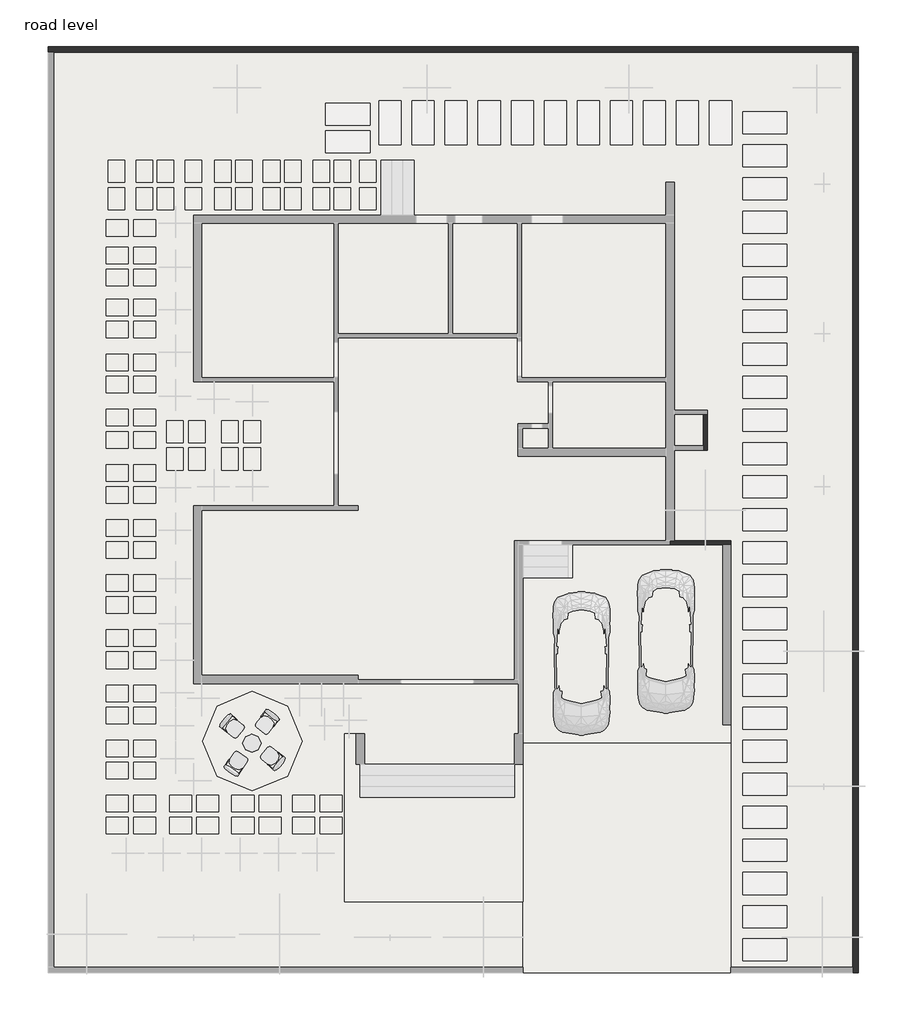
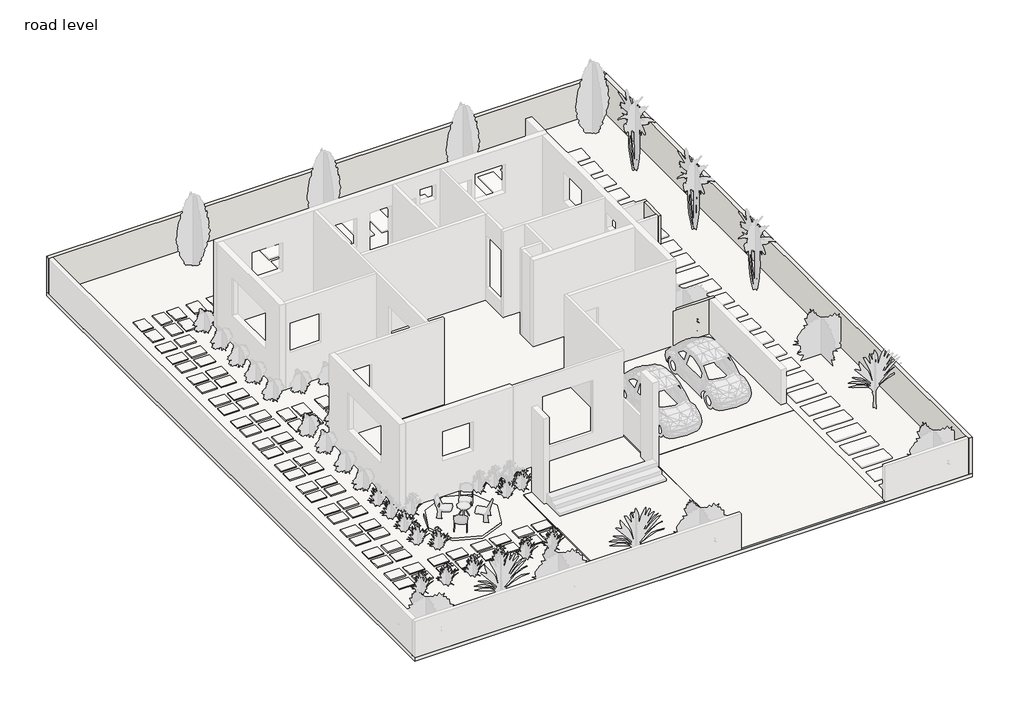
# One storey, part 2 of 3: 6 slabs, 4 walls.
"""IFC4 building model written with IfcOpenShell, lengths in millimetres."""

from ifc_helpers import new_model, si_unit, point, frame, frame_2d, origin, origin_with_axes, place, context, project, spatial, polyline, circle_curve, trimmed, segment, composite_curve, outline, extrude, faceted_brep, element, save

model = new_model("IFC4")

# Units and contexts
model_context = context("Model", 3, world=origin())
ifc_project = project(units=[si_unit("LENGTHUNIT", "METRE", prefix="MILLI")], contexts=[model_context])

# Site, building, storey
site = spatial("IfcSite", under=ifc_project)
building = spatial("IfcBuilding", under=site)
storey = spatial("IfcBuildingStorey", under=building, Name="road level", Elevation=0.0)

# Slabs
placement = place(None, origin())
element("IfcSlab", 1, ObjectType="Generic - 2\"", at=placement, inside=storey, context=model_context, shape_type="SweptSolid", body=[
    extrude(outline(polyline([(-8941.8271365, 12113.4780275), (-8941.8271365, 11503.8780275), (-9399.0271365, 11503.8780275), (-9399.0271365, 12113.4780275), (-8941.8271365, 12113.4780275)])), origin_with_axes(), (0.0, 0.0, 1.0), 50.8),
    extrude(outline(polyline([(-8941.8271365, 11355.5690245), (-8941.8271365, 10745.9690245), (-9399.0271365, 10745.9690245), (-9399.0271365, 11355.5690245), (-8941.8271365, 11355.5690245)])), origin_with_axes(), (0.0, 0.0, 1.0), 50.8),
    extrude(outline(polyline([(-9642.7719122, 12113.4780275), (-9642.7719122, 11503.8780275), (-10099.9719122, 11503.8780275), (-10099.9719122, 12113.4780275), (-9642.7719122, 12113.4780275)])), origin_with_axes(), (0.0, 0.0, 1.0), 50.8),
    extrude(outline(polyline([(-9642.7719122, 11355.5690245), (-9642.7719122, 10745.9690245), (-10099.9719122, 10745.9690245), (-10099.9719122, 11355.5690245), (-9642.7719122, 11355.5690245)])), origin_with_axes(), (0.0, 0.0, 1.0), 50.8),
    extrude(outline(polyline([(-10226.9719122, 12113.4780275), (-10226.9719122, 11503.8780275), (-10684.1719122, 11503.8780275), (-10684.1719122, 12113.4780275), (-10226.9719122, 12113.4780275)])), origin_with_axes(), (0.0, 0.0, 1.0), 50.8),
    extrude(outline(polyline([(-10226.9719122, 11355.5690245), (-10226.9719122, 10745.9690245), (-10684.1719122, 10745.9690245), (-10684.1719122, 11355.5690245), (-10226.9719122, 11355.5690245)])), origin_with_axes(), (0.0, 0.0, 1.0), 50.8),
    extrude(outline(polyline([(-11014.3719122, 12113.4780275), (-11014.3719122, 11503.8780275), (-11471.5719122, 11503.8780275), (-11471.5719122, 12113.4780275), (-11014.3719122, 12113.4780275)])), origin_with_axes(), (0.0, 0.0, 1.0), 50.8),
    extrude(outline(polyline([(-11014.3719122, 11355.5690245), (-11014.3719122, 10745.9690245), (-11471.5719122, 10745.9690245), (-11471.5719122, 11355.5690245), (-11014.3719122, 11355.5690245)])), origin_with_axes(), (0.0, 0.0, 1.0), 50.8),
    extrude(outline(polyline([(-11598.5719122, 12113.4780275), (-11598.5719122, 11503.8780275), (-12055.7719122, 11503.8780275), (-12055.7719122, 12113.4780275), (-11598.5719122, 12113.4780275)])), origin_with_axes(), (0.0, 0.0, 1.0), 50.8),
    extrude(outline(polyline([(-11598.5719122, 11355.5690245), (-11598.5719122, 10745.9690245), (-12055.7719122, 10745.9690245), (-12055.7719122, 11355.5690245), (-11598.5719122, 11355.5690245)])), origin_with_axes(), (0.0, 0.0, 1.0), 50.8),
    extrude(outline(polyline([(-12360.5719122, 12113.4780275), (-12360.5719122, 11503.8780275), (-12817.7719122, 11503.8780275), (-12817.7719122, 12113.4780275), (-12360.5719122, 12113.4780275)])), origin_with_axes(), (0.0, 0.0, 1.0), 50.8),
    extrude(outline(polyline([(-12360.5719122, 11355.5690245), (-12360.5719122, 10745.9690245), (-12817.7719122, 10745.9690245), (-12817.7719122, 11355.5690245), (-12360.5719122, 11355.5690245)])), origin_with_axes(), (0.0, 0.0, 1.0), 50.8),
    extrude(outline(polyline([(-12944.7719122, 12113.4780275), (-12944.7719122, 11503.8780275), (-13401.9719122, 11503.8780275), (-13401.9719122, 12113.4780275), (-12944.7719122, 12113.4780275)])), origin_with_axes(), (0.0, 0.0, 1.0), 50.8),
    extrude(outline(polyline([(-12944.7719122, 11355.5690245), (-12944.7719122, 10745.9690245), (-13401.9719122, 10745.9690245), (-13401.9719122, 11355.5690245), (-12944.7719122, 11355.5690245)])), origin_with_axes(), (0.0, 0.0, 1.0), 50.8),
    extrude(outline(polyline([(-13757.5719122, 12113.4780275), (-13757.5719122, 11503.8780275), (-14214.7719122, 11503.8780275), (-14214.7719122, 12113.4780275), (-13757.5719122, 12113.4780275)])), origin_with_axes(), (0.0, 0.0, 1.0), 50.8),
    extrude(outline(polyline([(-13757.5719122, 11355.5690245), (-13757.5719122, 10745.9690245), (-14214.7719122, 10745.9690245), (-14214.7719122, 11355.5690245), (-13757.5719122, 11355.5690245)])), origin_with_axes(), (0.0, 0.0, 1.0), 50.8),
    extrude(outline(polyline([(-14535.6391446, 12113.4780275), (-14535.6391446, 11503.8780275), (-14992.8391446, 11503.8780275), (-14992.8391446, 12113.4780275), (-14535.6391446, 12113.4780275)])), origin_with_axes(), (0.0, 0.0, 1.0), 50.8),
    extrude(outline(polyline([(-14535.6391446, 11355.5690245), (-14535.6391446, 10745.9690245), (-14992.8391446, 10745.9690245), (-14992.8391446, 11355.5690245), (-14535.6391446, 11355.5690245)])), origin_with_axes(), (0.0, 0.0, 1.0), 50.8),
    extrude(outline(polyline([(-15119.8391446, 12113.4780275), (-15119.8391446, 11503.8780275), (-15577.0391446, 11503.8780275), (-15577.0391446, 12113.4780275), (-15119.8391446, 12113.4780275)])), origin_with_axes(), (0.0, 0.0, 1.0), 50.8),
    extrude(outline(polyline([(-15119.8391446, 11355.5690245), (-15119.8391446, 10745.9690245), (-15577.0391446, 10745.9690245), (-15577.0391446, 11355.5690245), (-15119.8391446, 11355.5690245)])), origin_with_axes(), (0.0, 0.0, 1.0), 50.8),
    extrude(outline(polyline([(-15891.1719122, 12113.4780275), (-15891.1719122, 11503.8780275), (-16348.3719122, 11503.8780275), (-16348.3719122, 12113.4780275), (-15891.1719122, 12113.4780275)])), origin_with_axes(), (0.0, 0.0, 1.0), 50.8),
    extrude(outline(polyline([(-15891.1719122, 11355.5690245), (-15891.1719122, 10745.9690245), (-16348.3719122, 10745.9690245), (-16348.3719122, 11355.5690245), (-15891.1719122, 11355.5690245)])), origin_with_axes(), (0.0, 0.0, 1.0), 50.8),
    extrude(outline(polyline([(-15791.4182051, 10469.9168074), (-15791.4182051, 10012.7168074), (-16401.0182051, 10012.7168074), (-16401.0182051, 10469.9168074), (-15791.4182051, 10469.9168074)])), origin_with_axes(), (0.0, 0.0, 1.0), 50.8),
    extrude(outline(polyline([(-15033.5092021, 10469.9168074), (-15033.5092021, 10012.7168074), (-15643.1092021, 10012.7168074), (-15643.1092021, 10469.9168074), (-15033.5092021, 10469.9168074)])), origin_with_axes(), (0.0, 0.0, 1.0), 50.8),
    extrude(outline(polyline([(-15791.4182051, 9707.9168074), (-15791.4182051, 9250.7168074), (-16401.0182051, 9250.7168074), (-16401.0182051, 9707.9168074), (-15791.4182051, 9707.9168074)])), origin_with_axes(), (0.0, 0.0, 1.0), 50.8),
    extrude(outline(polyline([(-15033.5092021, 9707.9168074), (-15033.5092021, 9250.7168074), (-15643.1092021, 9250.7168074), (-15643.1092021, 9707.9168074), (-15033.5092021, 9707.9168074)])), origin_with_axes(), (0.0, 0.0, 1.0), 50.8),
    extrude(outline(polyline([(-15791.4182051, 9098.3168074), (-15791.4182051, 8641.1168074), (-16401.0182051, 8641.1168074), (-16401.0182051, 9098.3168074), (-15791.4182051, 9098.3168074)])), origin_with_axes(), (0.0, 0.0, 1.0), 50.8),
    extrude(outline(polyline([(-15033.5092021, 9098.3168074), (-15033.5092021, 8641.1168074), (-15643.1092021, 8641.1168074), (-15643.1092021, 9098.3168074), (-15033.5092021, 9098.3168074)])), origin_with_axes(), (0.0, 0.0, 1.0), 50.8),
    extrude(outline(polyline([(-15791.4182051, 8272.8168074), (-15791.4182051, 7815.6168074), (-16401.0182051, 7815.6168074), (-16401.0182051, 8272.8168074), (-15791.4182051, 8272.8168074)])), origin_with_axes(), (0.0, 0.0, 1.0), 50.8),
    extrude(outline(polyline([(-15033.5092021, 8272.8168074), (-15033.5092021, 7815.6168074), (-15643.1092021, 7815.6168074), (-15643.1092021, 8272.8168074), (-15033.5092021, 8272.8168074)])), origin_with_axes(), (0.0, 0.0, 1.0), 50.8),
    extrude(outline(polyline([(-15791.4182051, 7663.2168074), (-15791.4182051, 7206.0168074), (-16401.0182051, 7206.0168074), (-16401.0182051, 7663.2168074), (-15791.4182051, 7663.2168074)])), origin_with_axes(), (0.0, 0.0, 1.0), 50.8),
    extrude(outline(polyline([(-15033.5092021, 7663.2168074), (-15033.5092021, 7206.0168074), (-15643.1092021, 7206.0168074), (-15643.1092021, 7663.2168074), (-15033.5092021, 7663.2168074)])), origin_with_axes(), (0.0, 0.0, 1.0), 50.8),
    extrude(outline(polyline([(-15791.4182051, 6748.8168074), (-15791.4182051, 6291.6168074), (-16401.0182051, 6291.6168074), (-16401.0182051, 6748.8168074), (-15791.4182051, 6748.8168074)])), origin_with_axes(), (0.0, 0.0, 1.0), 50.8),
    extrude(outline(polyline([(-15033.5092021, 6748.8168074), (-15033.5092021, 6291.6168074), (-15643.1092021, 6291.6168074), (-15643.1092021, 6748.8168074), (-15033.5092021, 6748.8168074)])), origin_with_axes(), (0.0, 0.0, 1.0), 50.8),
    extrude(outline(polyline([(-15791.4182051, 6139.2168074), (-15791.4182051, 5682.0168074), (-16401.0182051, 5682.0168074), (-16401.0182051, 6139.2168074), (-15791.4182051, 6139.2168074)])), origin_with_axes(), (0.0, 0.0, 1.0), 50.8),
    extrude(outline(polyline([(-15033.5092021, 6139.2168074), (-15033.5092021, 5682.0168074), (-15643.1092021, 5682.0168074), (-15643.1092021, 6139.2168074), (-15033.5092021, 6139.2168074)])), origin_with_axes(), (0.0, 0.0, 1.0), 50.8),
    extrude(outline(polyline([(-15791.4182051, 5224.8168074), (-15791.4182051, 4767.6168074), (-16401.0182051, 4767.6168074), (-16401.0182051, 5224.8168074), (-15791.4182051, 5224.8168074)])), origin_with_axes(), (0.0, 0.0, 1.0), 50.8),
    extrude(outline(polyline([(-15033.5092021, 5224.8168074), (-15033.5092021, 4767.6168074), (-15643.1092021, 4767.6168074), (-15643.1092021, 5224.8168074), (-15033.5092021, 5224.8168074)])), origin_with_axes(), (0.0, 0.0, 1.0), 50.8),
    extrude(outline(polyline([(-15791.4182051, 4615.2168074), (-15791.4182051, 4158.0168074), (-16401.0182051, 4158.0168074), (-16401.0182051, 4615.2168074), (-15791.4182051, 4615.2168074)])), origin_with_axes(), (0.0, 0.0, 1.0), 50.8),
    extrude(outline(polyline([(-15033.5092021, 4615.2168074), (-15033.5092021, 4158.0168074), (-15643.1092021, 4158.0168074), (-15643.1092021, 4615.2168074), (-15033.5092021, 4615.2168074)])), origin_with_axes(), (0.0, 0.0, 1.0), 50.8),
    extrude(outline(polyline([(-15791.4182051, 3700.8168074), (-15791.4182051, 3243.6168074), (-16401.0182051, 3243.6168074), (-16401.0182051, 3700.8168074), (-15791.4182051, 3700.8168074)])), origin_with_axes(), (0.0, 0.0, 1.0), 50.8),
    extrude(outline(polyline([(-15033.5092021, 3700.8168074), (-15033.5092021, 3243.6168074), (-15643.1092021, 3243.6168074), (-15643.1092021, 3700.8168074), (-15033.5092021, 3700.8168074)])), origin_with_axes(), (0.0, 0.0, 1.0), 50.8),
    extrude(outline(polyline([(-15791.4182051, 3091.2168074), (-15791.4182051, 2634.0168074), (-16401.0182051, 2634.0168074), (-16401.0182051, 3091.2168074), (-15791.4182051, 3091.2168074)])), origin_with_axes(), (0.0, 0.0, 1.0), 50.8),
    extrude(outline(polyline([(-15033.5092021, 3091.2168074), (-15033.5092021, 2634.0168074), (-15643.1092021, 2634.0168074), (-15643.1092021, 3091.2168074), (-15033.5092021, 3091.2168074)])), origin_with_axes(), (0.0, 0.0, 1.0), 50.8),
    extrude(outline(polyline([(-15791.4182051, 2176.8168074), (-15791.4182051, 1719.6168074), (-16401.0182051, 1719.6168074), (-16401.0182051, 2176.8168074), (-15791.4182051, 2176.8168074)])), origin_with_axes(), (0.0, 0.0, 1.0), 50.8),
    extrude(outline(polyline([(-15033.5092021, 2176.8168074), (-15033.5092021, 1719.6168074), (-15643.1092021, 1719.6168074), (-15643.1092021, 2176.8168074), (-15033.5092021, 2176.8168074)])), origin_with_axes(), (0.0, 0.0, 1.0), 50.8),
    extrude(outline(polyline([(-15791.4182051, 1567.2168074), (-15791.4182051, 1110.0168074), (-16401.0182051, 1110.0168074), (-16401.0182051, 1567.2168074), (-15791.4182051, 1567.2168074)])), origin_with_axes(), (0.0, 0.0, 1.0), 50.8),
    extrude(outline(polyline([(-15033.5092021, 1567.2168074), (-15033.5092021, 1110.0168074), (-15643.1092021, 1110.0168074), (-15643.1092021, 1567.2168074), (-15033.5092021, 1567.2168074)])), origin_with_axes(), (0.0, 0.0, 1.0), 50.8),
    extrude(outline(polyline([(-15791.4182051, 652.8168074), (-15791.4182051, 195.6168074), (-16401.0182051, 195.6168074), (-16401.0182051, 652.8168074), (-15791.4182051, 652.8168074)])), origin_with_axes(), (0.0, 0.0, 1.0), 50.8),
    extrude(outline(polyline([(-15033.5092021, 652.8168074), (-15033.5092021, 195.6168074), (-15643.1092021, 195.6168074), (-15643.1092021, 652.8168074), (-15033.5092021, 652.8168074)])), origin_with_axes(), (0.0, 0.0, 1.0), 50.8),
    extrude(outline(polyline([(-15791.4182051, 43.2168074), (-15791.4182051, -413.9831926), (-16401.0182051, -413.9831926), (-16401.0182051, 43.2168074), (-15791.4182051, 43.2168074)])), origin_with_axes(), (0.0, 0.0, 1.0), 50.8),
    extrude(outline(polyline([(-15033.5092021, 43.2168074), (-15033.5092021, -413.9831926), (-15643.1092021, -413.9831926), (-15643.1092021, 43.2168074), (-15033.5092021, 43.2168074)])), origin_with_axes(), (0.0, 0.0, 1.0), 50.8),
    extrude(outline(polyline([(-15791.4182051, -871.1831926), (-15791.4182051, -1328.3831926), (-16401.0182051, -1328.3831926), (-16401.0182051, -871.1831926), (-15791.4182051, -871.1831926)])), origin_with_axes(), (0.0, 0.0, 1.0), 50.8),
    extrude(outline(polyline([(-15033.5092021, -871.1831926), (-15033.5092021, -1328.3831926), (-15643.1092021, -1328.3831926), (-15643.1092021, -871.1831926), (-15033.5092021, -871.1831926)])), origin_with_axes(), (0.0, 0.0, 1.0), 50.8),
    extrude(outline(polyline([(-15791.4182051, -1480.7831926), (-15791.4182051, -1937.9831926), (-16401.0182051, -1937.9831926), (-16401.0182051, -1480.7831926), (-15791.4182051, -1480.7831926)])), origin_with_axes(), (0.0, 0.0, 1.0), 50.8),
    extrude(outline(polyline([(-15033.5092021, -1480.7831926), (-15033.5092021, -1937.9831926), (-15643.1092021, -1937.9831926), (-15643.1092021, -1480.7831926), (-15033.5092021, -1480.7831926)])), origin_with_axes(), (0.0, 0.0, 1.0), 50.8),
    extrude(outline(polyline([(-15791.4182051, -2395.1831926), (-15791.4182051, -2852.3831926), (-16401.0182051, -2852.3831926), (-16401.0182051, -2395.1831926), (-15791.4182051, -2395.1831926)])), origin_with_axes(), (0.0, 0.0, 1.0), 50.8),
    extrude(outline(polyline([(-15033.5092021, -2395.1831926), (-15033.5092021, -2852.3831926), (-15643.1092021, -2852.3831926), (-15643.1092021, -2395.1831926), (-15033.5092021, -2395.1831926)])), origin_with_axes(), (0.0, 0.0, 1.0), 50.8),
    extrude(outline(polyline([(-15791.4182051, -3004.7831926), (-15791.4182051, -3461.9831926), (-16401.0182051, -3461.9831926), (-16401.0182051, -3004.7831926), (-15791.4182051, -3004.7831926)])), origin_with_axes(), (0.0, 0.0, 1.0), 50.8),
    extrude(outline(polyline([(-15033.5092021, -3004.7831926), (-15033.5092021, -3461.9831926), (-15643.1092021, -3461.9831926), (-15643.1092021, -3004.7831926), (-15033.5092021, -3004.7831926)])), origin_with_axes(), (0.0, 0.0, 1.0), 50.8),
    extrude(outline(polyline([(-15791.4182051, -3919.1831926), (-15791.4182051, -4376.3831926), (-16401.0182051, -4376.3831926), (-16401.0182051, -3919.1831926), (-15791.4182051, -3919.1831926)])), origin_with_axes(), (0.0, 0.0, 1.0), 50.8),
    extrude(outline(polyline([(-15033.5092021, -3919.1831926), (-15033.5092021, -4376.3831926), (-15643.1092021, -4376.3831926), (-15643.1092021, -3919.1831926), (-15033.5092021, -3919.1831926)])), origin_with_axes(), (0.0, 0.0, 1.0), 50.8),
    extrude(outline(polyline([(-15791.4182051, -4528.7831926), (-15791.4182051, -4985.9831926), (-16401.0182051, -4985.9831926), (-16401.0182051, -4528.7831926), (-15791.4182051, -4528.7831926)])), origin_with_axes(), (0.0, 0.0, 1.0), 50.8),
    extrude(outline(polyline([(-15033.5092021, -4528.7831926), (-15033.5092021, -4985.9831926), (-15643.1092021, -4985.9831926), (-15643.1092021, -4528.7831926), (-15033.5092021, -4528.7831926)])), origin_with_axes(), (0.0, 0.0, 1.0), 50.8),
    extrude(outline(polyline([(-15791.4182051, -5443.1831926), (-15791.4182051, -5900.3831926), (-16401.0182051, -5900.3831926), (-16401.0182051, -5443.1831926), (-15791.4182051, -5443.1831926)])), origin_with_axes(), (0.0, 0.0, 1.0), 50.8),
    extrude(outline(polyline([(-15033.5092021, -5443.1831926), (-15033.5092021, -5900.3831926), (-15643.1092021, -5900.3831926), (-15643.1092021, -5443.1831926), (-15033.5092021, -5443.1831926)])), origin_with_axes(), (0.0, 0.0, 1.0), 50.8),
    extrude(outline(polyline([(-15791.4182051, -6052.7831926), (-15791.4182051, -6509.9831926), (-16401.0182051, -6509.9831926), (-16401.0182051, -6052.7831926), (-15791.4182051, -6052.7831926)])), origin_with_axes(), (0.0, 0.0, 1.0), 50.8),
    extrude(outline(polyline([(-15033.5092021, -6052.7831926), (-15033.5092021, -6509.9831926), (-15643.1092021, -6509.9831926), (-15643.1092021, -6052.7831926), (-15033.5092021, -6052.7831926)])), origin_with_axes(), (0.0, 0.0, 1.0), 50.8),
    extrude(outline(polyline([(-14043.9871576, -5443.1831926), (-14043.9871576, -5900.3831926), (-14653.5871576, -5900.3831926), (-14653.5871576, -5443.1831926), (-14043.9871576, -5443.1831926)])), origin_with_axes(), (0.0, 0.0, 1.0), 50.8),
    extrude(outline(polyline([(-14043.9871576, -6052.7831926), (-14043.9871576, -6509.9831926), (-14653.5871576, -6509.9831926), (-14653.5871576, -6052.7831926), (-14043.9871576, -6052.7831926)])), origin_with_axes(), (0.0, 0.0, 1.0), 50.8),
    extrude(outline(polyline([(-13286.0781547, -5443.1831926), (-13286.0781547, -5900.3831926), (-13895.6781547, -5900.3831926), (-13895.6781547, -5443.1831926), (-13286.0781547, -5443.1831926)])), origin_with_axes(), (0.0, 0.0, 1.0), 50.8),
    extrude(outline(polyline([(-13286.0781547, -6052.7831926), (-13286.0781547, -6509.9831926), (-13895.6781547, -6509.9831926), (-13895.6781547, -6052.7831926), (-13286.0781547, -6052.7831926)])), origin_with_axes(), (0.0, 0.0, 1.0), 50.8),
    extrude(outline(polyline([(-12316.7871576, -5443.1831926), (-12316.7871576, -5900.3831926), (-12926.3871576, -5900.3831926), (-12926.3871576, -5443.1831926), (-12316.7871576, -5443.1831926)])), origin_with_axes(), (0.0, 0.0, 1.0), 50.8),
    extrude(outline(polyline([(-12316.7871576, -6052.7831926), (-12316.7871576, -6509.9831926), (-12926.3871576, -6509.9831926), (-12926.3871576, -6052.7831926), (-12316.7871576, -6052.7831926)])), origin_with_axes(), (0.0, 0.0, 1.0), 50.8),
    extrude(outline(polyline([(-11558.8781547, -5443.1831926), (-11558.8781547, -5900.3831926), (-12168.4781547, -5900.3831926), (-12168.4781547, -5443.1831926), (-11558.8781547, -5443.1831926)])), origin_with_axes(), (0.0, 0.0, 1.0), 50.8),
    extrude(outline(polyline([(-11558.8781547, -6052.7831926), (-11558.8781547, -6509.9831926), (-12168.4781547, -6509.9831926), (-12168.4781547, -6052.7831926), (-11558.8781547, -6052.7831926)])), origin_with_axes(), (0.0, 0.0, 1.0), 50.8),
    extrude(outline(polyline([(-14271.6721908, 4917.9713089), (-14271.6721908, 4308.3713089), (-14728.8721908, 4308.3713089), (-14728.8721908, 4917.9713089), (-14271.6721908, 4917.9713089)])), origin_with_axes(), (0.0, 0.0, 1.0), 50.8),
    extrude(outline(polyline([(-13662.0721908, 4917.9713089), (-13662.0721908, 4308.3713089), (-14119.2721908, 4308.3713089), (-14119.2721908, 4917.9713089), (-13662.0721908, 4917.9713089)])), origin_with_axes(), (0.0, 0.0, 1.0), 50.8),
    extrude(outline(polyline([(-14271.6721908, 4160.0623059), (-14271.6721908, 3550.4623059), (-14728.8721908, 3550.4623059), (-14728.8721908, 4160.0623059), (-14271.6721908, 4160.0623059)])), origin_with_axes(), (0.0, 0.0, 1.0), 50.8),
    extrude(outline(polyline([(-13662.0721908, 4160.0623059), (-13662.0721908, 3550.4623059), (-14119.2721908, 3550.4623059), (-14119.2721908, 4160.0623059), (-13662.0721908, 4160.0623059)])), origin_with_axes(), (0.0, 0.0, 1.0), 50.8),
    extrude(outline(polyline([(-12747.6721908, 4917.9713089), (-12747.6721908, 4308.3713089), (-13204.8721908, 4308.3713089), (-13204.8721908, 4917.9713089), (-12747.6721908, 4917.9713089)])), origin_with_axes(), (0.0, 0.0, 1.0), 50.8),
    extrude(outline(polyline([(-12138.0721908, 4917.9713089), (-12138.0721908, 4308.3713089), (-12595.2721908, 4308.3713089), (-12595.2721908, 4917.9713089), (-12138.0721908, 4917.9713089)])), origin_with_axes(), (0.0, 0.0, 1.0), 50.8),
    extrude(outline(polyline([(-12747.6721908, 4160.0623059), (-12747.6721908, 3550.4623059), (-13204.8721908, 3550.4623059), (-13204.8721908, 4160.0623059), (-12747.6721908, 4160.0623059)])), origin_with_axes(), (0.0, 0.0, 1.0), 50.8),
    extrude(outline(polyline([(-12138.0721908, 4160.0623059), (-12138.0721908, 3550.4623059), (-12595.2721908, 3550.4623059), (-12595.2721908, 4160.0623059), (-12138.0721908, 4160.0623059)])), origin_with_axes(), (0.0, 0.0, 1.0), 50.8),
    extrude(outline(polyline([(-10640.3871576, -5443.1831926), (-10640.3871576, -5900.3831926), (-11249.9871576, -5900.3831926), (-11249.9871576, -5443.1831926), (-10640.3871576, -5443.1831926)])), origin_with_axes(), (0.0, 0.0, 1.0), 50.8),
    extrude(outline(polyline([(-10640.3871576, -6052.7831926), (-10640.3871576, -6509.9831926), (-11249.9871576, -6509.9831926), (-11249.9871576, -6052.7831926), (-10640.3871576, -6052.7831926)])), origin_with_axes(), (0.0, 0.0, 1.0), 50.8),
    extrude(outline(polyline([(-9882.4781547, -5443.1831926), (-9882.4781547, -5900.3831926), (-10492.0781547, -5900.3831926), (-10492.0781547, -5443.1831926), (-9882.4781547, -5443.1831926)])), origin_with_axes(), (0.0, 0.0, 1.0), 50.8),
    extrude(outline(polyline([(-9882.4781547, -6052.7831926), (-9882.4781547, -6509.9831926), (-10492.0781547, -6509.9831926), (-10492.0781547, -6052.7831926), (-9882.4781547, -6052.7831926)])), origin_with_axes(), (0.0, 0.0, 1.0), 50.8),
])
element("IfcSlab", 2, ObjectType="Generic - 2\" 2", at=placement, inside=storey, context=model_context, shape_type="SweptSolid", body=[
    extrude(outline(polyline([(-9807.8719122, -3741.3831926), (-9490.3719122, -3741.3831926), (-9490.3719122, -4585.9331926), (-4879.4781622, -4585.9331926), (-4879.4781622, -8389.5831926), (-9807.8719122, -8389.5831926), (-9807.8719122, -3741.3831926)])), origin_with_axes(), (0.0, 0.0, 1.0), 50.8),
])
element("IfcSlab", 3, ObjectType="Generic - 2\" 2", at=placement, inside=storey, context=model_context, shape_type="SweptSolid", body=[
    extrude(outline(polyline([(879.1780878, -10344.6627683), (-4879.4781622, -10344.6627683), (-4879.4781622, -4001.0127683), (879.1780878, -4001.0127683), (879.1780878, -10344.6627683)])), origin_with_axes(), (0.0, 0.0, 1.0), 50.8),
])
element("IfcSlab", 4, ObjectType="Generic - 6\" 2", at=placement, inside=storey, context=model_context, shape_type="SweptSolid", body=[
    extrude(outline(polyline([(879.1780878, 1595.7918074), (879.1780878, -4004.9081926), (-4994.5719122, -4004.9081926), (-4994.5719122, 1595.7918074), (879.1780878, 1595.7918074)])), origin_with_axes(), (0.0, 0.0, 1.0), 50.8),
])
element("IfcSlab", 5, ObjectType="Generic - 6\" 4", at=placement, inside=storey, context=model_context, shape_type="SweptSolid", body=[
    extrude(outline(polyline([(4400.3423756, 15258.5372317), (4400.3423756, -10344.6627683), (-18008.8076244, -10344.6627683), (-18008.8076244, 15258.5372317), (4400.3423756, 15258.5372317)])), frame((0.0, 0.0, -152.4), z_axis=(0.0, 0.0, 1.0), x_axis=(1.0, 0.0, 0.0)), (0.0, 0.0, 1.0), 152.4),
])
element("IfcSlab", 6, ObjectType="Generic - 6\" 6", at=placement, inside=storey, context=model_context, shape_type="SweptSolid", body=[
    extrude(outline(composite_curve([segment(trimmed(circle_curve(frame_2d((-12361.4832026, -3944.5831926)), 1371.6), [point((-13733.0832026, -3944.5831926))], [point((-10989.8832026, -3944.5831926))], False, "CARTESIAN"), True, "CONTINUOUS"), segment(trimmed(circle_curve(frame_2d((-12361.4832026, -3944.5831926)), 1371.6), [point((-10989.8832026, -3944.5831926))], [point((-13733.0832026, -3944.5831926))], False, "CARTESIAN"), True, "CONTINUOUS")], self_intersect=False)), frame((0.0, 0.0, 50.8), z_axis=(0.0, 0.0, 1.0), x_axis=(1.0, 0.0, 0.0)), (0.0, 0.0, 1.0), 101.6),
])

# Walls
element("IfcWall", 7, ObjectType="Generic - 4.5\"", at=placement, inside=storey, context=model_context, shape_type="Brep", body=[
    faceted_brep([(-803.5719122, 1481.4918074, 0.0), (650.5780878, 1481.4918074, 0.0), (879.1780878, 1481.4918074, 0.0), (879.1780878, 1481.4918074, 1524.0), (650.5780878, 1481.4918074, 1524.0), (-689.2719122, 1481.4918074, 1524.0), (-803.5719122, 1481.4918074, 1524.0), (-803.5719122, 1595.7918074, 0.0), (-803.5719122, 1595.7918074, 1524.0), (-689.2719122, 1595.7918074, 1524.0), (879.1780878, 1595.7918074, 1524.0), (879.1780878, 1595.7918074, 0.0), (-689.2719122, 1595.7918074, 0.0)], [[[0, 1, 2, 3, 4, 5, 6]], [[7, 8, 9, 10, 11, 12]], [[2, 1, 0, 7, 12, 11]], [[6, 5, 4, 3, 10, 9, 8]], [[0, 6, 8, 7]], [[3, 2, 11, 10]]]),
])
element("IfcWall", 8, ObjectType="Generic - 4.5\"", at=placement, inside=storey, context=model_context, shape_type="Brep", body=[
    faceted_brep([(117.1780878, 5091.4668074, 0.0), (117.1780878, 4215.1668074, 0.0), (117.1780878, 4100.8668074, 0.0), (117.1780878, 4100.8668074, 3657.6), (117.1780878, 4215.1668074, 3657.6), (117.1780878, 5091.4668074, 3657.6), (231.4780878, 5091.4668074, 0.0), (231.4780878, 5091.4668074, 3657.6), (231.4780878, 4100.8668074, 3657.6), (231.4780878, 4100.8668074, 0.0)], [[[0, 1, 2, 3, 4, 5]], [[6, 7, 8, 9]], [[2, 1, 0, 6, 9]], [[5, 4, 3, 8, 7]], [[0, 5, 7, 6]], [[3, 2, 9, 8]]]),
])
element("IfcWall", 9, ObjectType="Generic - 6\"", at=placement, inside=storey, context=model_context, shape_type="Brep", body=[
    faceted_brep([(-18002.4576244, 15106.1372317, 0.0), (-17850.0576244, 15106.1372317, 0.0), (4247.9423756, 15106.1372317, 0.0), (4400.3423756, 15106.1372317, 0.0), (4400.3423756, 15106.1372317, 1524.0), (4247.9423756, 15106.1372317, 1524.0), (-17850.0576244, 15106.1372317, 1524.0), (-18002.4576244, 15106.1372317, 1524.0), (-18002.4576244, 15258.5372317, 0.0), (-18002.4576244, 15258.5372317, 1524.0), (4400.3423756, 15258.5372317, 1524.0), (4400.3423756, 15258.5372317, 0.0)], [[[0, 1, 2, 3, 4, 5, 6, 7]], [[8, 9, 10, 11]], [[3, 2, 1, 0, 8, 11]], [[7, 6, 5, 4, 10, 9]], [[4, 3, 11, 10]], [[0, 7, 9, 8]]]),
])
element("IfcWall", 10, ObjectType="Generic - 6\"", at=placement, inside=storey, context=model_context, shape_type="Brep", body=[
    faceted_brep([(4247.9423756, 15106.1372317, 0.0), (4247.9423756, -10192.2627683, 0.0), (4247.9423756, -10344.6627683, 0.0), (4247.9423756, -10344.6627683, 1524.0), (4247.9423756, -10192.2627683, 1524.0), (4247.9423756, 15106.1372317, 1524.0), (4400.3423756, 15106.1372317, 0.0), (4400.3423756, 15106.1372317, 1524.0), (4400.3423756, -10344.6627683, 1524.0), (4400.3423756, -10344.6627683, 0.0)], [[[0, 1, 2, 3, 4, 5]], [[6, 7, 8, 9]], [[2, 1, 0, 6, 9]], [[5, 4, 3, 8, 7]], [[0, 5, 7, 6]], [[3, 2, 9, 8]]]),
])

save(model, "model.ifc")

# Revit data of these elements
# Type "Generic - 2\""
#   Assembly Code = "B1010"
#   Function = 0
#   Layers, outside or top first: 0' - 2" "Tile, Mosaic, Gray" (function 1)
# Type "Generic - 2\" 2"
#   Assembly Code = "B1010"
#   Function = 0
#   Layers, outside or top first: 0' - 2" "Concrete, Precast" (function 1)
# Type "Generic - 6\" 2"
#   Assembly Code = "B1010"
#   Function = 0
#   Layers, outside or top first: 0' - 2" no material (function 1)
# Type "Generic - 6\" 4"
#   Assembly Code = "B1010"
#   Function = 0
#   Layers, outside or top first: 0' - 6" "Grass" (function 1)
# Type "Generic - 6\" 6"
#   Assembly Code = "B1010"
#   Function = 0
#   Layers, outside or top first: 0' - 4" "Wood - Teak" (function 1)
# Type "Generic - 4.5\""
#   Assembly Code = "B2010"
#   Layers, outside or top first: 0' - 4 1/2" no material (function 1)
# Type "Generic - 6\""
#   Assembly Code = "B2010"
#   Layers, outside or top first: 0' - 6" no material (function 1)
# Element 1 (IfcSlab, "Generic - 2\"")
#   Height Offset From Level = 0' - 2"
#   Phase Created = New Construction
#   Materials on its faces: "Tile, Mosaic, Gray"
# Element 2 (IfcSlab, "Generic - 2\" 2")
#   built-in parameter 1001955 = 3.14159 (stored number, unit not read)
#   Height Offset From Level = 0' - 2"
#   Phase Created = New Construction
#   Materials on its faces: "Concrete, Precast"
# Element 3 (IfcSlab, "Generic - 2\" 2")
#   built-in parameter 1001955 = -1.5708 (stored number, unit not read)
#   Height Offset From Level = 0' - 2"
#   Phase Created = New Construction
#   Materials on its faces: "Concrete, Precast"
# Element 4 (IfcSlab, "Generic - 6\" 2")
#   Height Offset From Level = 0' - 2"
#   Phase Created = New Construction
#   Materials on its faces: "Default Floor"
# Element 5 (IfcSlab, "Generic - 6\" 4")
#   Height Offset From Level = 0' - 0"
#   Phase Created = New Construction
#   Materials on its faces: "Grass"
# Element 6 (IfcSlab, "Generic - 6\" 6")
#   Height Offset From Level = 0' - 6"
#   Phase Created = New Construction
#   Materials on its faces: "Wood - Teak"
# Element 7 (IfcWall, "Generic - 4.5\"")
#   Top Offset = 0' - 0"
#   Base Offset = 0' - 0"
#   Unconnected Height = 5' - 0"
#   wall height = 5' - 0"
#   Phase Created = New Construction
#   Base Constraint = road level
#   Materials on its faces: "Default Wall"
# Element 8 (IfcWall, "Generic - 4.5\"")
#   Top Offset = 0' - 0"
#   Base Offset = 0' - 0"
#   wall height = 12' - 0"
#   Phase Created = New Construction
#   Base Constraint = road level
#   Top Constraint = terrace
#   Materials on its faces: "Default Wall"
# Elements 9, 10 (IfcWall, "Generic - 6\"")
#   Top Offset = 0' - 0"
#   Base Offset = 0' - 0"
#   Unconnected Height = 5' - 0"
#   wall height = 5' - 0"
#   Phase Created = New Construction
#   Base Constraint = road level
#   Materials on its faces: "Default Wall"
# Materials
#   "Tile, Mosaic, Gray": class "Generic", colour RGB 127 127 127, transparency 0, Description = "Mosiac tile, gray", Cost = 0
#   "Concrete, Precast": class "Concrete", colour RGB 198 187 187, transparency 0, Description = "Precast concrete", Cost = 0
#   "Grass": class "Generic", colour RGB 104 137 66, transparency 0, Description = "Physical material.", Cost = 0
#   "Wood - Teak": colour RGB 150 100 26, transparency 0
#   "Default Floor": colour RGB 128 128 128, transparency 0, Cost = 0
#   "Default Wall": colour RGB 128 128 128, transparency 0, Cost = 0
